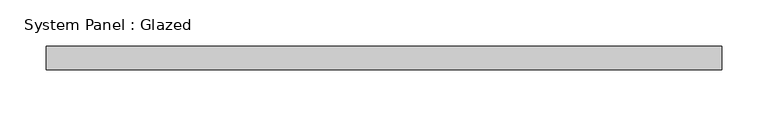
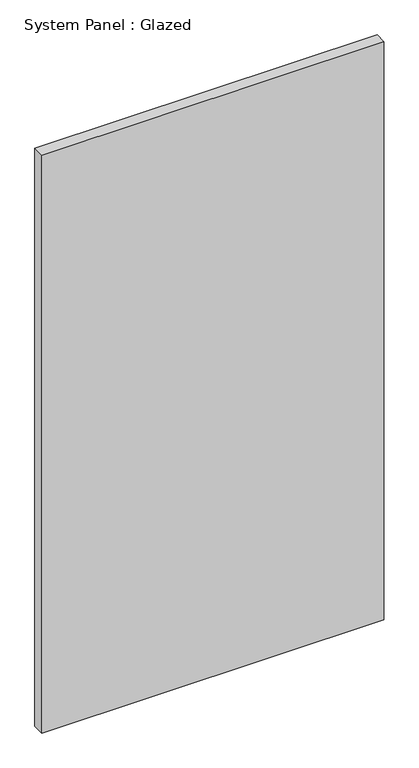
"""IFC4 building model written with IfcOpenShell, lengths in millimetres: plate geometry, System Panel : Glazed."""

from ifc_helpers import new_model, si_unit, origin, origin_with_axes, place, context, project, spatial, polyline, outline, extrude, source, transform, mapped, element, save


def system_panel_glazed_05e8e754(model_context):
    return source(origin(), model_context, "Body", "SweptSolid", [
        extrude(outline(polyline([(366.1833333, 19.05), (-366.1833333, 19.05), (-366.1833333, 44.45), (366.1833333, 44.45), (366.1833333, 19.05)])), origin_with_axes(), (0.0, 0.0, 1.0), 1308.1),
    ])


if __name__ == "__main__":
    model = new_model("IFC4")
    model_context = context("Model", 3, world=origin())
    ifc_project = project(units=[si_unit("LENGTHUNIT", "METRE", prefix="MILLI")], contexts=[model_context])
    site = spatial("IfcSite", under=ifc_project)
    building = spatial("IfcBuilding", under=site)
    placement = place(None, origin())
    system_panel_glazed_shape = system_panel_glazed_05e8e754(model_context)
    element("IfcPlate", 1, ObjectType="System Panel : Glazed", at=placement, inside=building, context=model_context, shape_type="MappedRepresentation", body=[
        mapped(system_panel_glazed_shape, transform((0.0, 0.0, 0.0), x_axis=(1.0, 0.0, 0.0), y_axis=(0.0, 1.0, 0.0), z_axis=(0.0, 0.0, 1.0))),
    ])
    save(model, "model.ifc")

# Revit data of these elements
# Type "System Panel : Glazed"
#   Construction Type Id = "GSP4R"
#   Analytic Construction = "1/8 in Pilkington single glazing"
#   Visual Light Transmittance = 0.9
#   Solar Heat Gain Coefficient = 0.86
#   Heat Transfer Coefficient (U) = 1.18115 BTU/(h·ft²·°F)
# Element 1 (IfcPlate, "System Panel : Glazed")
#   Materials on its faces: "Glass"
# Materials
#   "Glass": class "Glass", colour RGB 0 128 192, transparency 0.75, Description = "Soda Lime Glass", Cost = 0
